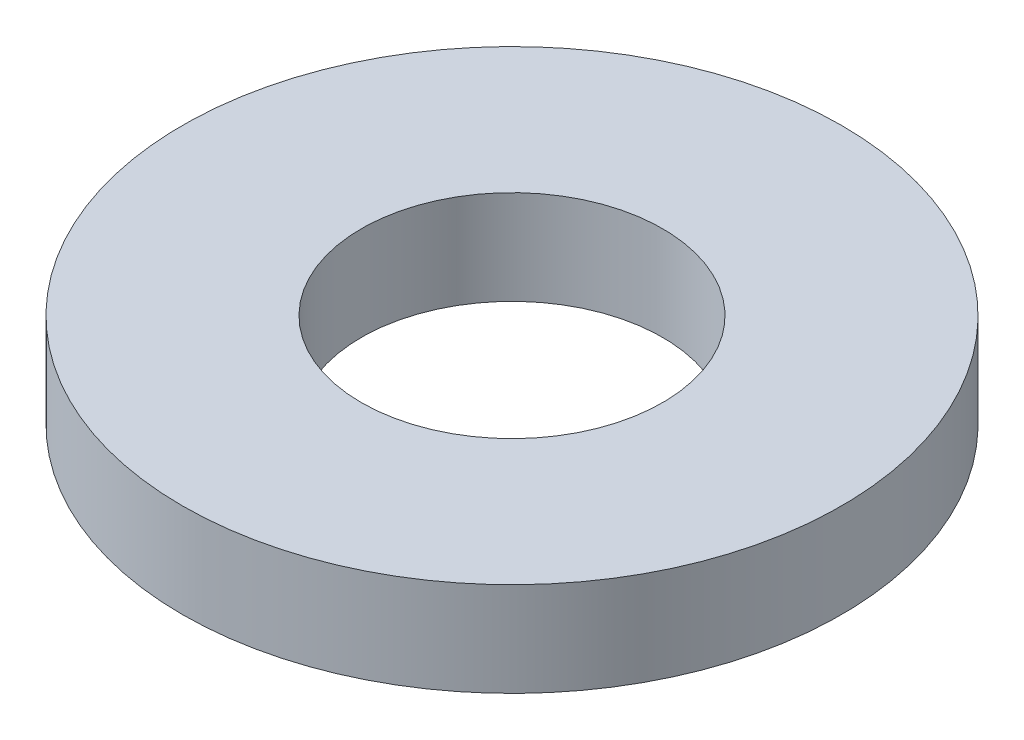
from build123d import *

# Parameters (mm, degrees)
WASHER_PROFILE_35_16_R   = 17.5
WASHER_PROFILE_35_16_R_2 = 8
WASHER_BODY_5MM_DEPTH    = 2.5


with BuildPart() as part:
    # Washer Profile Ø35-Ø16 → Washer Body 5mm (new, symmetric)
    with BuildSketch(Plane(origin=(0, 0, 0), x_dir=(1, 0, 0), z_dir=(0, 1, 0))):
        with Locations(Location((0, 0, 0), (0, 0, 270))):
            Circle(WASHER_PROFILE_35_16_R)
        with Locations(Location((0, 0, 0), (0, 0, 270))):
            Circle(WASHER_PROFILE_35_16_R_2, mode=Mode.SUBTRACT)
    extrude(amount=WASHER_BODY_5MM_DEPTH, both=True)


solid = part.part
